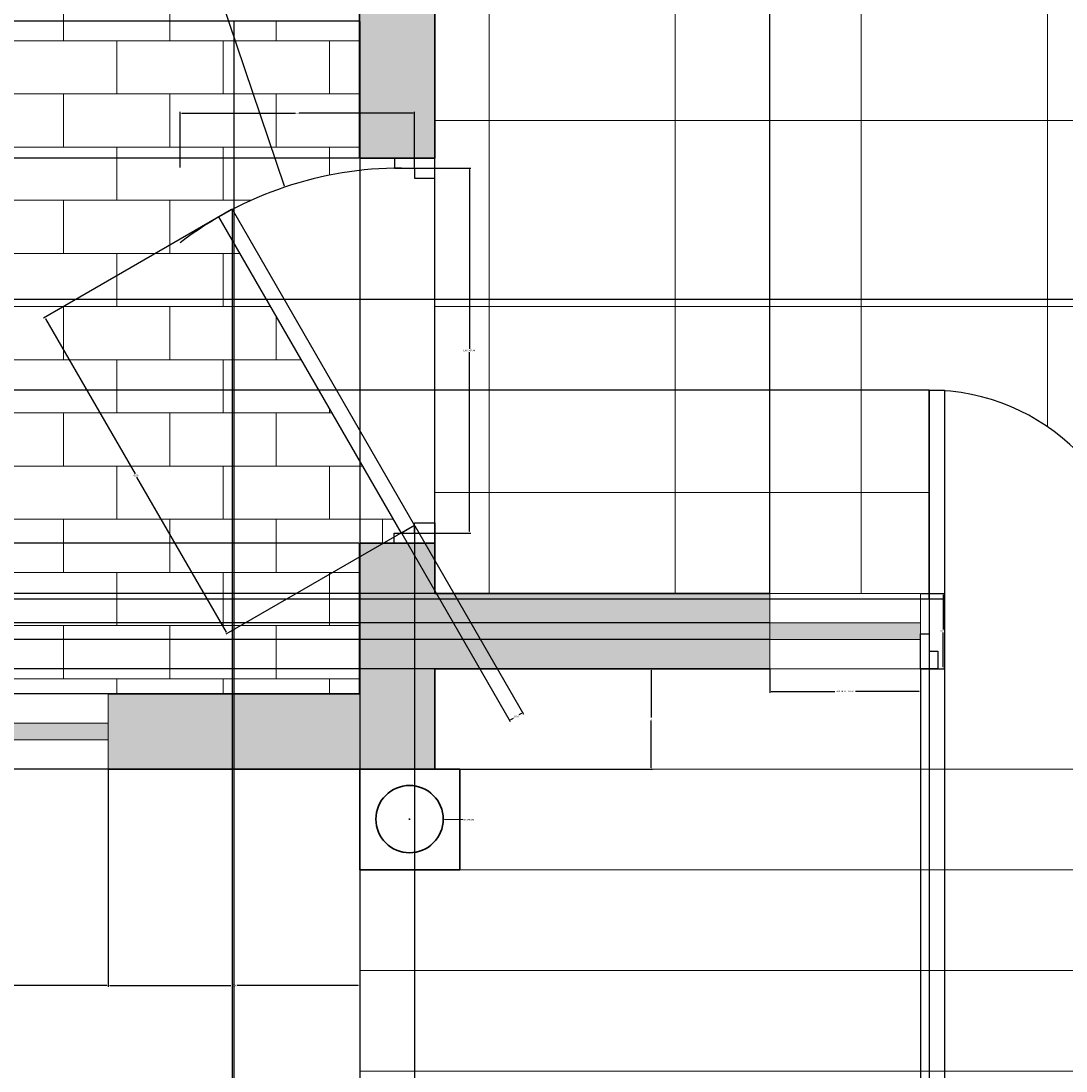
# Model space of a CAD drawing. Units: inches. Extents: x 6 to 575, y 34 to 566.
# Tile 4 of 21: x 157 to 282, y 168 to 293. Entities that reach past the tile are written whole.
import ezdxf

# ---------------------------------------------------------------- set-up
doc = ezdxf.new("R2010")
doc.units = ezdxf.units.IN
doc.linetypes.add('ACAD_ISO02W100', pattern=[15, 12, -3])
for name, color, linetype, lineweight in [('A-ANNO-DIMS', 2, 'Continuous', 18), ('A-COLS', 7, 'Continuous', 35), ('A-DOOR-THRS', 8, 'Continuous', 13), ('A-FLOR-PATT', 252, 'Continuous', 9), ('A-GLAZ-PATT', 4, 'Continuous', 9), ('A-ROOF-OVHD', 240, 'ACAD_ISO02W100', 13), ('A-WALL-PATT', 251, 'Continuous', 9), ('DOORS', 3, 'Continuous', 25), ('STAIRS', 1, 'Continuous', 20), ('WALLS', 7, 'Continuous', 35), ('WINDOWS', 4, 'Continuous', 20)]:
    doc.layers.add(name, color=color, linetype=linetype, lineweight=lineweight)
doc.styles.get("Standard").update_dxf_attribs({"font": 'arial.ttf'})
doc.dimstyles.get("Standard").update_dxf_attribs({"dimtxt": 0.18, "dimasz": 0.18, "dimexe": 0.18, "dimexo": 0.0625, "dimgap": 0.09, "dimtad": 0, "dimtih": 1, "dimtoh": 1, "dimdec": 4, "dimzin": 0, "dimdsep": 46, "dimtxsty": 'Standard', "dimcen": 0.09, "dimadec": 0, "dimazin": 0, "dimtfac": 1, "dimtdec": 4, "dimtofl": 0, "dimtmove": 0, "dimatfit": 3, "dimfxl": 1, "dimtolj": 1, "dimtzin": 0, "dimarcsym": 0})

# ---------------------------------------------------------------- blocks, each defined once
blk = doc.blocks.new('Door - Left Hung 36 in.')
blk.add_lwpolyline([(0.75, -1.3), (0, 0), (31.18, 18), (31.93, 16.7)], close=True)
blk.add_arc((0, 0), 36, 0, 37.3101)
blk = doc.blocks.new('*U4')
for p, q in [((0, 0), (0, -6)), ((24, 0), (24, -6))]:
    blk.add_line(p, q)
blk.add_lwpolyline([(0, 0), (0, 24), (1.75, 24), (1.75, 0)], close=True)
blk.add_arc((0, 0), 24, 0, 90)
blk = doc.blocks.new('WIN-SIDELIGHT-18IN')
for p, q in [((0, 9), (0, 0)), ((0, 0), (0, 9)), ((0, 9), (0, 0)), ((18, 9), (18, 0)), ((0, 5.5), (18, 5.5)), ((0, 3.5), (18, 3.5))]:
    blk.add_line(p, q)
blk.add_lwpolyline([(0, 9), (18, 9), (18, 0), (0, 0)], close=True)
blk = doc.blocks.new('COL-PORTICO-RECT-BASE')
blk.add_lwpolyline([(0, 12.01), (11.94, 12.01), (11.94, 0), (0, 0)], close=True)
blk.add_circle((5.95, 6.05), 4.02)
blk = doc.blocks.new('*D15')
at = {"layer": 'A-ANNO-DIMS', "color": 0, "lineweight": -2, "transparency": 16777216}
for p, q in [((204.3, 275.6), (210.96, 275.6)), ((210.78, 275.42), (210.78, 253.99)), ((210.78, 232.19), (210.78, 253.62)), ((204.3, 232.01), (210.96, 232.01))]:
    blk.add_line(p, q, dxfattribs=at)
at = {"layer": 'A-ANNO-DIMS', "color": 0, "transparency": 16777216}
for points in [[(210.75, 275.42), (210.81, 275.42), (210.78, 275.6)], [(210.75, 232.19), (210.81, 232.19), (210.78, 232.01)]]:
    blk.add_solid(points, dxfattribs=at)
at = {"layer": 'Defpoints', "color": 0, "transparency": 16777216}
for p in [(204.24, 275.6), (210.78, 275.6), (204.24, 232.01)]:
    blk.add_point(p, dxfattribs=at)
at = {"layer": 'A-ANNO-DIMS', "color": 0, "transparency": 16777216, "insert": (210.78, 253.81), "char_height": 0.18, "attachment_point": 5}
blk.add_mtext('\\A1;LH DOOR 44', dxfattribs=at)
blk = doc.blocks.new('*D16')
at = {"layer": 'A-ANNO-DIMS', "color": 0, "lineweight": -2, "transparency": 16777216}
for p, q in [((176.25, 275.66), (176.25, 282.32)), ((204.24, 275.66), (204.24, 282.32)), ((176.43, 282.14), (190.02, 282.14)), ((204.06, 282.14), (190.46, 282.14))]:
    blk.add_line(p, q, dxfattribs=at)
at = {"layer": 'A-ANNO-DIMS', "color": 0, "transparency": 16777216}
for points in [[(176.43, 282.17), (176.43, 282.11), (176.25, 282.14)], [(204.06, 282.17), (204.06, 282.11), (204.24, 282.14)]]:
    blk.add_solid(points, dxfattribs=at)
at = {"layer": 'Defpoints', "color": 0, "transparency": 16777216}
for p in [(176.25, 282.14), (176.25, 275.6), (204.24, 275.6)]:
    blk.add_point(p, dxfattribs=at)
at = {"layer": 'A-ANNO-DIMS', "color": 0, "transparency": 16777216, "insert": (190.24, 282.14), "char_height": 0.18, "attachment_point": 5}
blk.add_mtext('\\A1;28', dxfattribs=at)
blk = doc.blocks.new('*D19')
at = {"layer": 'A-ANNO-DIMS', "color": 0, "lineweight": -2, "transparency": 16777216}
for p, q in [((246.66, 215.74), (246.66, 212.92)), ((264.66, 215.74), (264.66, 212.92)), ((246.84, 213.1), (254.43, 213.1)), ((264.48, 213.1), (256.88, 213.1))]:
    blk.add_line(p, q, dxfattribs=at)
at = {"layer": 'A-ANNO-DIMS', "color": 0, "transparency": 16777216}
for points in [[(246.84, 213.13), (246.84, 213.07), (246.66, 213.1)], [(264.48, 213.13), (264.48, 213.07), (264.66, 213.1)]]:
    blk.add_solid(points, dxfattribs=at)
at = {"layer": 'Defpoints', "color": 0, "transparency": 16777216}
for p in [(246.66, 215.8), (264.66, 215.8), (264.66, 213.1)]:
    blk.add_point(p, dxfattribs=at)
at = {"layer": 'A-ANNO-DIMS', "color": 0, "transparency": 16777216, "insert": (255.66, 213.1), "char_height": 0.18, "attachment_point": 5}
blk.add_mtext('\\A1;SIDELIGHT 18 TYP.', dxfattribs=at)
blk = doc.blocks.new('*D20')
at = {"layer": 'A-ANNO-DIMS', "color": 0, "lineweight": -2, "transparency": 16777216}
for p, q in [((264.72, 224.8), (267.54, 224.8)), ((267.36, 224.62), (267.36, 220.48)), ((267.36, 215.98), (267.36, 220.12)), ((264.72, 215.8), (267.54, 215.8))]:
    blk.add_line(p, q, dxfattribs=at)
at = {"layer": 'A-ANNO-DIMS', "color": 0, "transparency": 16777216}
for points in [[(267.33, 224.62), (267.39, 224.62), (267.36, 224.8)], [(267.33, 215.98), (267.39, 215.98), (267.36, 215.8)]]:
    blk.add_solid(points, dxfattribs=at)
at = {"layer": 'Defpoints', "color": 0, "transparency": 16777216}
for p in [(264.66, 224.8), (267.36, 224.8), (264.66, 215.8)]:
    blk.add_point(p, dxfattribs=at)
at = {"layer": 'A-ANNO-DIMS', "color": 0, "transparency": 16777216, "insert": (267.36, 220.3), "char_height": 0.18, "attachment_point": 5}
blk.add_mtext('\\A1;9 TYP.', dxfattribs=at)
blk = doc.blocks.new('*D29')
at = {"layer": 'A-ANNO-DIMS', "color": 0, "lineweight": -2, "transparency": 16777216}
for p, q in [((32.66, 203.74), (32.66, 33.76)), ((548.66, 203.74), (548.66, 33.76)), ((32.84, 33.94), (290.37, 33.94)), ((548.48, 33.94), (290.95, 33.94))]:
    blk.add_line(p, q, dxfattribs=at)
at = {"layer": 'A-ANNO-DIMS', "color": 0, "transparency": 16777216}
for points in [[(32.84, 33.97), (32.84, 33.91), (32.66, 33.94)], [(548.48, 33.97), (548.48, 33.91), (548.66, 33.94)]]:
    blk.add_solid(points, dxfattribs=at)
at = {"layer": 'Defpoints', "color": 0, "transparency": 16777216}
for p in [(32.66, 203.8), (548.66, 203.8), (548.66, 33.94)]:
    blk.add_point(p, dxfattribs=at)
at = {"layer": 'A-ANNO-DIMS', "color": 0, "transparency": 16777216, "insert": (290.66, 33.94), "char_height": 0.18, "attachment_point": 5}
blk.add_mtext('\\A1;516', dxfattribs=at)
blk = doc.blocks.new('*D30')
at = {"layer": 'A-ANNO-DIMS', "color": 0, "lineweight": -2, "transparency": 16777216}
for p, q in [((32.6, 539.8), (6.65, 539.8)), ((6.83, 539.62), (6.83, 299.97)), ((6.83, 59.95), (6.83, 299.61)), ((197.62, 59.77), (6.65, 59.77))]:
    blk.add_line(p, q, dxfattribs=at)
at = {"layer": 'A-ANNO-DIMS', "color": 0, "transparency": 16777216}
for points in [[(6.8, 539.62), (6.86, 539.62), (6.83, 539.8)], [(6.8, 59.95), (6.86, 59.95), (6.83, 59.77)]]:
    blk.add_solid(points, dxfattribs=at)
at = {"layer": 'Defpoints', "color": 0, "transparency": 16777216}
for p in [(32.66, 539.8), (6.83, 59.77), (197.69, 59.77)]:
    blk.add_point(p, dxfattribs=at)
at = {"layer": 'A-ANNO-DIMS', "color": 0, "transparency": 16777216, "insert": (6.83, 299.79), "char_height": 0.18, "attachment_point": 5}
blk.add_mtext('\\A1;480', dxfattribs=at)
blk = doc.blocks.new('*D37')
at = {"layer": 'A-ANNO-DIMS', "color": 0, "lineweight": -2, "transparency": 16777216}
for p, q in [((71.66, 203.74), (71.66, 177.79)), ((167.66, 203.74), (167.66, 177.79)), ((71.84, 177.97), (119.44, 177.97)), ((167.48, 177.97), (119.88, 177.97))]:
    blk.add_line(p, q, dxfattribs=at)
at = {"layer": 'A-ANNO-DIMS', "color": 0, "transparency": 16777216}
for points in [[(71.84, 178), (71.84, 177.94), (71.66, 177.97)], [(167.48, 178), (167.48, 177.94), (167.66, 177.97)]]:
    blk.add_solid(points, dxfattribs=at)
at = {"layer": 'Defpoints', "color": 0, "transparency": 16777216}
for p in [(71.66, 203.8), (167.66, 203.8), (71.66, 177.97)]:
    blk.add_point(p, dxfattribs=at)
at = {"layer": 'A-ANNO-DIMS', "color": 0, "transparency": 16777216, "insert": (119.66, 177.97), "char_height": 0.18, "attachment_point": 5}
blk.add_mtext('\\A1;96', dxfattribs=at)
blk = doc.blocks.new('*D39')
at = {"layer": 'A-ANNO-DIMS', "color": 0, "lineweight": -2, "transparency": 16777216}
for p, q in [((167.66, 203.74), (167.66, 177.79)), ((197.69, 203.74), (197.69, 177.79)), ((167.84, 177.97), (182.28, 177.97)), ((197.51, 177.97), (183.07, 177.97))]:
    blk.add_line(p, q, dxfattribs=at)
at = {"layer": 'A-ANNO-DIMS', "color": 0, "transparency": 16777216}
for points in [[(167.84, 178), (167.84, 177.94), (167.66, 177.97)], [(197.51, 178), (197.51, 177.94), (197.69, 177.97)]]:
    blk.add_solid(points, dxfattribs=at)
at = {"layer": 'Defpoints', "color": 0, "transparency": 16777216}
for p in [(167.66, 203.8), (197.69, 203.8), (167.66, 177.97)]:
    blk.add_point(p, dxfattribs=at)
at = {"layer": 'A-ANNO-DIMS', "color": 0, "transparency": 16777216, "insert": (182.67, 177.97), "char_height": 0.18, "attachment_point": 5}
blk.add_mtext('\\A1;30.03', dxfattribs=at)
blk = doc.blocks.new('*D48')
at = {"layer": 'A-ANNO-DIMS', "color": 0, "lineweight": -2, "transparency": 16777216}
for p, q in [((264.66, 215.74), (264.66, 33.76)), ((316.66, 215.74), (316.66, 33.76)), ((264.84, 33.94), (290.44, 33.94)), ((316.48, 33.94), (290.88, 33.94))]:
    blk.add_line(p, q, dxfattribs=at)
at = {"layer": 'A-ANNO-DIMS', "color": 0, "transparency": 16777216}
for points in [[(264.84, 33.97), (264.84, 33.91), (264.66, 33.94)], [(316.48, 33.97), (316.48, 33.91), (316.66, 33.94)]]:
    blk.add_solid(points, dxfattribs=at)
at = {"layer": 'Defpoints', "color": 0, "transparency": 16777216}
for p in [(264.66, 215.8), (316.66, 215.8), (316.66, 33.94)]:
    blk.add_point(p, dxfattribs=at)
at = {"layer": 'A-ANNO-DIMS', "color": 0, "transparency": 16777216, "insert": (290.66, 33.94), "char_height": 0.18, "attachment_point": 5}
blk.add_mtext('\\A1;52', dxfattribs=at)
blk = doc.blocks.new('*D54')
at = {"layer": 'A-ANNO-DIMS', "color": 0, "lineweight": -2, "transparency": 16777216}
for p, q in [((444.96, 337.94), (6.65, 337.94)), ((6.83, 337.76), (6.83, 299.11)), ((6.83, 260.1), (6.83, 298.75)), ((444.96, 259.92), (6.65, 259.92))]:
    blk.add_line(p, q, dxfattribs=at)
at = {"layer": 'A-ANNO-DIMS', "color": 0, "transparency": 16777216}
for points in [[(6.8, 337.76), (6.86, 337.76), (6.83, 337.94)], [(6.8, 260.1), (6.86, 260.1), (6.83, 259.92)]]:
    blk.add_solid(points, dxfattribs=at)
at = {"layer": 'Defpoints', "color": 0, "transparency": 16777216}
for p in [(6.83, 337.94), (445.02, 337.94), (445.02, 259.92)]:
    blk.add_point(p, dxfattribs=at)
at = {"layer": 'A-ANNO-DIMS', "color": 0, "transparency": 16777216, "insert": (6.83, 298.93), "char_height": 0.18, "attachment_point": 5}
blk.add_mtext('\\A1;78.02', dxfattribs=at)
blk = doc.blocks.new('*D59')
at = {"layer": 'A-ANNO-DIMS', "color": 0, "lineweight": -2, "transparency": 16777216}
for p, q in [((206.66, 224.86), (206.66, 565.81)), ((206.84, 565.63), (226.44, 565.63)), ((246.48, 565.63), (226.88, 565.63)), ((246.66, 224.86), (246.66, 565.81))]:
    blk.add_line(p, q, dxfattribs=at)
at = {"layer": 'A-ANNO-DIMS', "color": 0, "transparency": 16777216}
for points in [[(206.84, 565.66), (206.84, 565.6), (206.66, 565.63)], [(246.48, 565.66), (246.48, 565.6), (246.66, 565.63)]]:
    blk.add_solid(points, dxfattribs=at)
at = {"layer": 'Defpoints', "color": 0, "transparency": 16777216}
for p in [(246.66, 565.63), (206.66, 224.8), (246.66, 224.8)]:
    blk.add_point(p, dxfattribs=at)
at = {"layer": 'A-ANNO-DIMS', "color": 0, "transparency": 16777216, "insert": (226.66, 565.63), "char_height": 0.18, "attachment_point": 5}
blk.add_mtext('\\A1;40', dxfattribs=at)
blk = doc.blocks.new('*D60')
at = {"layer": 'A-ANNO-DIMS', "color": 0, "lineweight": -2, "transparency": 16777216}
for p, q in [((206.72, 215.8), (232.67, 215.8)), ((232.49, 215.62), (232.49, 209.98)), ((232.49, 203.98), (232.49, 209.62)), ((206.72, 203.8), (232.67, 203.8))]:
    blk.add_line(p, q, dxfattribs=at)
at = {"layer": 'A-ANNO-DIMS', "color": 0, "transparency": 16777216}
for points in [[(232.46, 215.62), (232.52, 215.62), (232.49, 215.8)], [(232.46, 203.98), (232.52, 203.98), (232.49, 203.8)]]:
    blk.add_solid(points, dxfattribs=at)
at = {"layer": 'Defpoints', "color": 0, "transparency": 16777216}
for p in [(206.66, 215.8), (206.66, 203.8), (232.49, 203.8)]:
    blk.add_point(p, dxfattribs=at)
at = {"layer": 'A-ANNO-DIMS', "color": 0, "transparency": 16777216, "insert": (232.49, 209.8), "char_height": 0.18, "attachment_point": 5}
blk.add_mtext('\\A1;12', dxfattribs=at)
blk = doc.blocks.new('*D77')
at = {"layer": 'A-ANNO-DIMS', "color": 0, "lineweight": -2, "transparency": 16777216}
for p, q in [((197.62, 203.8), (6.65, 203.8)), ((6.83, 203.62), (6.83, 131.97)), ((6.83, 59.95), (6.83, 131.61)), ((197.62, 59.77), (6.65, 59.77))]:
    blk.add_line(p, q, dxfattribs=at)
at = {"layer": 'A-ANNO-DIMS', "color": 0, "transparency": 16777216}
for points in [[(6.8, 203.62), (6.86, 203.62), (6.83, 203.8)], [(6.8, 59.95), (6.86, 59.95), (6.83, 59.77)]]:
    blk.add_solid(points, dxfattribs=at)
at = {"layer": 'Defpoints', "color": 0, "transparency": 16777216}
for p in [(6.83, 203.8), (197.69, 203.8), (197.69, 59.77)]:
    blk.add_point(p, dxfattribs=at)
at = {"layer": 'A-ANNO-DIMS', "color": 0, "transparency": 16777216, "insert": (6.83, 131.79), "char_height": 0.18, "attachment_point": 5}
blk.add_mtext('\\A1;144.03', dxfattribs=at)
blk = doc.blocks.new('*D104')
at = {"layer": 'A-ANNO-DIMS', "color": 0, "lineweight": -2, "transparency": 16777216}
for p, q in [((197.64, 348.32), (6.65, 348.32)), ((6.83, 348.14), (6.83, 320.93)), ((6.83, 293.34), (6.83, 320.56)), ((182.58, 293.16), (6.65, 293.16))]:
    blk.add_line(p, q, dxfattribs=at)
at = {"layer": 'A-ANNO-DIMS', "color": 0, "transparency": 16777216}
for points in [[(6.8, 348.14), (6.86, 348.14), (6.83, 348.32)], [(6.8, 293.34), (6.86, 293.34), (6.83, 293.16)]]:
    blk.add_solid(points, dxfattribs=at)
at = {"layer": 'Defpoints', "color": 0, "transparency": 16777216}
for p in [(6.83, 348.32), (197.7, 348.32), (182.64, 293.16)]:
    blk.add_point(p, dxfattribs=at)
at = {"layer": 'A-ANNO-DIMS', "color": 0, "transparency": 16777216, "insert": (6.83, 320.74), "char_height": 0.18, "attachment_point": 5}
blk.add_mtext('\\A1;55.16', dxfattribs=at)
blk = doc.blocks.new('*D105')
at = {"layer": 'A-ANNO-DIMS', "color": 0, "lineweight": -2, "transparency": 16777216}
for p, q in [((182.64, 293.1), (182.64, 33.76)), ((197.7, 293.1), (197.7, 33.76)), ((182.82, 33.94), (189.71, 33.94)), ((197.52, 33.94), (190.62, 33.94))]:
    blk.add_line(p, q, dxfattribs=at)
at = {"layer": 'A-ANNO-DIMS', "color": 0, "transparency": 16777216}
for points in [[(182.82, 33.97), (182.82, 33.91), (182.64, 33.94)], [(197.52, 33.97), (197.52, 33.91), (197.7, 33.94)]]:
    blk.add_solid(points, dxfattribs=at)
at = {"layer": 'Defpoints', "color": 0, "transparency": 16777216}
for p in [(182.64, 293.16), (197.7, 293.16), (197.7, 33.94)]:
    blk.add_point(p, dxfattribs=at)
at = {"layer": 'A-ANNO-DIMS', "color": 0, "transparency": 16777216, "insert": (190.17, 33.94), "char_height": 0.18, "attachment_point": 5}
blk.add_mtext('\\A1;15.058', dxfattribs=at)
blk = doc.blocks.new('*D106')
at = {"layer": 'A-ANNO-DIMS', "color": 0, "lineweight": -2, "transparency": 16777216}
for p, q in [((197.64, 293.16), (6.65, 293.16)), ((6.83, 292.98), (6.83, 285.16)), ((6.83, 276.98), (6.83, 284.8)), ((197.6, 276.8), (6.65, 276.8))]:
    blk.add_line(p, q, dxfattribs=at)
at = {"layer": 'A-ANNO-DIMS', "color": 0, "transparency": 16777216}
for points in [[(6.8, 292.98), (6.86, 292.98), (6.83, 293.16)], [(6.8, 276.98), (6.86, 276.98), (6.83, 276.8)]]:
    blk.add_solid(points, dxfattribs=at)
at = {"layer": 'Defpoints', "color": 0, "transparency": 16777216}
for p in [(6.83, 293.16), (197.7, 293.16), (197.66, 276.8)]:
    blk.add_point(p, dxfattribs=at)
at = {"layer": 'A-ANNO-DIMS', "color": 0, "transparency": 16777216, "insert": (6.83, 284.98), "char_height": 0.18, "attachment_point": 5}
blk.add_mtext('\\A1;16.363', dxfattribs=at)
blk = doc.blocks.new('*D107')
at = {"layer": 'A-ANNO-DIMS', "color": 0, "lineweight": -2, "transparency": 16777216}
for p, q in [((197.6, 230.8), (6.65, 230.8)), ((6.83, 230.62), (6.83, 221.98)), ((6.83, 212.98), (6.83, 221.62)), ((197.6, 212.8), (6.65, 212.8))]:
    blk.add_line(p, q, dxfattribs=at)
at = {"layer": 'A-ANNO-DIMS', "color": 0, "transparency": 16777216}
for points in [[(6.8, 230.62), (6.86, 230.62), (6.83, 230.8)], [(6.8, 212.98), (6.86, 212.98), (6.83, 212.8)]]:
    blk.add_solid(points, dxfattribs=at)
at = {"layer": 'Defpoints', "color": 0, "transparency": 16777216}
for p in [(6.83, 230.8), (197.66, 230.8), (197.66, 212.8)]:
    blk.add_point(p, dxfattribs=at)
at = {"layer": 'A-ANNO-DIMS', "color": 0, "transparency": 16777216, "insert": (6.83, 221.8), "char_height": 0.18, "attachment_point": 5}
blk.add_mtext('\\A1;18', dxfattribs=at)
blk = doc.blocks.new('*D108')
at = {"layer": 'A-ANNO-DIMS', "color": 0, "lineweight": -2, "transparency": 16777216}
for p, q in [((197.6, 276.8), (6.65, 276.8)), ((6.83, 276.62), (6.83, 253.98)), ((6.83, 230.98), (6.83, 253.62)), ((197.6, 230.8), (6.65, 230.8))]:
    blk.add_line(p, q, dxfattribs=at)
at = {"layer": 'A-ANNO-DIMS', "color": 0, "transparency": 16777216}
for points in [[(6.8, 276.62), (6.86, 276.62), (6.83, 276.8)], [(6.8, 230.98), (6.86, 230.98), (6.83, 230.8)]]:
    blk.add_solid(points, dxfattribs=at)
at = {"layer": 'Defpoints', "color": 0, "transparency": 16777216}
for p in [(6.83, 276.8), (197.66, 276.8), (197.66, 230.8)]:
    blk.add_point(p, dxfattribs=at)
at = {"layer": 'A-ANNO-DIMS', "color": 0, "transparency": 16777216, "insert": (6.83, 253.8), "char_height": 0.18, "attachment_point": 5}
blk.add_mtext('\\A1;46', dxfattribs=at)
blk = doc.blocks.new('*D137')
at = {"layer": 'A-ANNO-DIMS', "color": 0, "lineweight": -2, "transparency": 16777216}
for p, q in [((206.62, 310.57), (6.65, 310.57)), ((6.83, 310.39), (6.83, 267.87)), ((6.83, 224.98), (6.83, 267.5)), ((206.6, 224.8), (6.65, 224.8))]:
    blk.add_line(p, q, dxfattribs=at)
at = {"layer": 'A-ANNO-DIMS', "color": 0, "transparency": 16777216}
for points in [[(6.8, 310.39), (6.86, 310.39), (6.83, 310.57)], [(6.8, 224.98), (6.86, 224.98), (6.83, 224.8)]]:
    blk.add_solid(points, dxfattribs=at)
at = {"layer": 'Defpoints', "color": 0, "transparency": 16777216}
for p in [(6.83, 310.57), (206.68, 310.57), (206.66, 224.8)]:
    blk.add_point(p, dxfattribs=at)
at = {"layer": 'A-ANNO-DIMS', "color": 0, "transparency": 16777216, "insert": (6.83, 267.69), "char_height": 0.18, "attachment_point": 5}
blk.add_mtext('\\A1;85.77', dxfattribs=at)
blk = doc.blocks.new('*D206')
at = {"layer": 'A-ANNO-DIMS', "color": 0, "lineweight": -2, "transparency": 16777216}
for p, q in [((182.39, 270.64), (159.92, 257.66)), ((160.16, 257.6), (170.87, 239.06)), ((181.78, 220.16), (171.08, 238.7)), ((204.18, 232.89), (181.71, 219.91))]:
    blk.add_line(p, q, dxfattribs=at)
at = {"layer": 'A-ANNO-DIMS', "color": 0, "transparency": 16777216}
for points in [[(160.19, 257.61), (160.14, 257.58), (160.07, 257.75)], [(181.8, 220.18), (181.75, 220.15), (181.87, 220)]]:
    blk.add_solid(points, dxfattribs=at)
at = {"layer": 'Defpoints', "color": 0, "transparency": 16777216}
for p in [(182.44, 270.67), (160.07, 257.75), (204.24, 232.92)]:
    blk.add_point(p, dxfattribs=at)
at = {"layer": 'A-ANNO-DIMS', "color": 0, "transparency": 16777216, "insert": (170.97, 238.88), "char_height": 0.18, "attachment_point": 5}
blk.add_mtext('\\A1;43.59', dxfattribs=at)
blk = doc.blocks.new('*D207')
at = {"layer": 'A-ANNO-DIMS', "color": 0, "lineweight": -2, "transparency": 16777216}
for p, q in [((204.27, 232.87), (217.24, 210.39)), ((202.7, 231.96), (215.67, 209.49)), ((215.74, 209.73), (216.05, 209.91)), ((217, 210.46), (216.68, 210.28))]:
    blk.add_line(p, q, dxfattribs=at)
at = {"layer": 'A-ANNO-DIMS', "color": 0, "transparency": 16777216}
for points in [[(215.72, 209.76), (215.75, 209.71), (215.58, 209.64)], [(216.98, 210.49), (217.01, 210.43), (217.15, 210.55)]]:
    blk.add_solid(points, dxfattribs=at)
at = {"layer": 'Defpoints', "color": 0, "transparency": 16777216}
for p in [(202.66, 232.01), (204.24, 232.92), (215.58, 209.64)]:
    blk.add_point(p, dxfattribs=at)
at = {"layer": 'A-ANNO-DIMS', "color": 0, "transparency": 16777216, "insert": (216.37, 210.1), "char_height": 0.18, "attachment_point": 5}
blk.add_mtext('\\A1;1.816', dxfattribs=at)
blk = doc.blocks.new('*D208')
at = {"layer": 'A-ANNO-DIMS', "color": 0, "lineweight": -2, "transparency": 16777216}
for p, q in [((182.44, 270.6), (182.44, 33.76)), ((204.24, 232.86), (204.24, 33.76)), ((182.62, 33.94), (192.88, 33.94)), ((204.06, 33.94), (193.81, 33.94))]:
    blk.add_line(p, q, dxfattribs=at)
at = {"layer": 'A-ANNO-DIMS', "color": 0, "transparency": 16777216}
for points in [[(182.62, 33.97), (182.62, 33.91), (182.44, 33.94)], [(204.06, 33.97), (204.06, 33.91), (204.24, 33.94)]]:
    blk.add_solid(points, dxfattribs=at)
at = {"layer": 'Defpoints', "color": 0, "transparency": 16777216}
for p in [(182.44, 270.67), (204.24, 232.92), (182.44, 33.94)]:
    blk.add_point(p, dxfattribs=at)
at = {"layer": 'A-ANNO-DIMS', "color": 0, "transparency": 16777216, "insert": (193.34, 33.94), "char_height": 0.18, "attachment_point": 5}
blk.add_mtext('\\A1;21.793', dxfattribs=at)
blk = doc.blocks.new('*D209')
at = {"layer": 'A-ANNO-DIMS', "color": 0, "lineweight": -2, "transparency": 16777216}
for p, q in [((265.64, 249.08), (6.65, 249.08)), ((6.83, 248.9), (6.83, 236.78)), ((6.83, 224.3), (6.83, 236.42)), ((265.64, 224.12), (6.65, 224.12))]:
    blk.add_line(p, q, dxfattribs=at)
at = {"layer": 'A-ANNO-DIMS', "color": 0, "transparency": 16777216}
for points in [[(6.8, 248.9), (6.86, 248.9), (6.83, 249.08)], [(6.8, 224.3), (6.86, 224.3), (6.83, 224.12)]]:
    blk.add_solid(points, dxfattribs=at)
at = {"layer": 'Defpoints', "color": 0, "transparency": 16777216}
for p in [(6.83, 249.08), (265.7, 249.08), (265.7, 224.12)]:
    blk.add_point(p, dxfattribs=at)
at = {"layer": 'A-ANNO-DIMS', "color": 0, "transparency": 16777216, "insert": (6.83, 236.6), "char_height": 0.18, "attachment_point": 5}
blk.add_mtext('\\A1;24.96', dxfattribs=at)
blk = doc.blocks.new('*D210')
at = {"layer": 'A-ANNO-DIMS', "color": 0, "lineweight": -2, "transparency": 16777216}
for p, q in [((265.7, 249.02), (265.7, 33.76)), ((267.52, 249.02), (267.52, 33.76)), ((265.88, 33.94), (266.29, 33.94)), ((267.34, 33.94), (266.92, 33.94))]:
    blk.add_line(p, q, dxfattribs=at)
at = {"layer": 'A-ANNO-DIMS', "color": 0, "transparency": 16777216}
for points in [[(265.88, 33.97), (265.88, 33.91), (265.7, 33.94)], [(267.34, 33.97), (267.34, 33.91), (267.52, 33.94)]]:
    blk.add_solid(points, dxfattribs=at)
at = {"layer": 'Defpoints', "color": 0, "transparency": 16777216}
for p in [(265.7, 249.08), (267.52, 249.08), (267.52, 33.94)]:
    blk.add_point(p, dxfattribs=at)
at = {"layer": 'A-ANNO-DIMS', "color": 0, "transparency": 16777216, "insert": (266.61, 33.94), "char_height": 0.18, "attachment_point": 5}
blk.add_mtext('\\A1;1.82', dxfattribs=at)
blk = doc.blocks.new('*D214')
at = {"layer": 'A-ANNO-DIMS', "color": 0, "lineweight": -2, "transparency": 16777216}
for p, q in [((246.6, 219.3), (6.65, 219.3)), ((6.83, 219.12), (6.83, 217.73)), ((6.83, 215.98), (6.83, 217.37)), ((246.6, 215.8), (6.65, 215.8))]:
    blk.add_line(p, q, dxfattribs=at)
at = {"layer": 'A-ANNO-DIMS', "color": 0, "transparency": 16777216}
for points in [[(6.8, 219.12), (6.86, 219.12), (6.83, 219.3)], [(6.8, 215.98), (6.86, 215.98), (6.83, 215.8)]]:
    blk.add_solid(points, dxfattribs=at)
at = {"layer": 'Defpoints', "color": 0, "transparency": 16777216}
for p in [(6.83, 219.3), (246.66, 219.3), (246.66, 215.8)]:
    blk.add_point(p, dxfattribs=at)
at = {"layer": 'A-ANNO-DIMS', "color": 0, "transparency": 16777216, "insert": (6.83, 217.55), "char_height": 0.18, "attachment_point": 5}
blk.add_mtext('\\A1;3.5', dxfattribs=at)
blk = doc.blocks.new('*D215')
at = {"layer": 'A-ANNO-DIMS', "color": 0, "lineweight": -2, "transparency": 16777216}
for p, q in [((246.6, 221.3), (6.65, 221.3)), ((6.83, 221.12), (6.83, 220.48)), ((6.83, 219.48), (6.83, 220.12)), ((246.6, 219.3), (6.65, 219.3))]:
    blk.add_line(p, q, dxfattribs=at)
at = {"layer": 'A-ANNO-DIMS', "color": 0, "transparency": 16777216}
for points in [[(6.8, 221.12), (6.86, 221.12), (6.83, 221.3)], [(6.8, 219.48), (6.86, 219.48), (6.83, 219.3)]]:
    blk.add_solid(points, dxfattribs=at)
at = {"layer": 'Defpoints', "color": 0, "transparency": 16777216}
for p in [(6.83, 221.3), (246.66, 221.3), (246.66, 219.3)]:
    blk.add_point(p, dxfattribs=at)
at = {"layer": 'A-ANNO-DIMS', "color": 0, "transparency": 16777216, "insert": (6.83, 220.3), "char_height": 0.18, "attachment_point": 5}
blk.add_mtext('\\A1;2', dxfattribs=at)
blk = doc.blocks.new('*D219')
at = {"layer": 'A-ANNO-DIMS', "color": 0, "lineweight": -2, "transparency": 16777216}
for p, q in [((203.54, 197.84), (203.72, 197.84)), ((203.63, 197.75), (203.63, 197.93)), ((210.06, 197.76), (207.83, 197.79))]:
    blk.add_line(p, q, dxfattribs=at)
at = {"layer": 'A-ANNO-DIMS', "color": 0, "transparency": 16777216}
blk.add_solid([(207.83, 197.82), (207.83, 197.76), (207.65, 197.79)], dxfattribs=at)
at = {"layer": 'Defpoints', "color": 0, "transparency": 16777216}
for p in [(199.62, 197.89), (207.65, 197.79)]:
    blk.add_point(p, dxfattribs=at)
at = {"layer": 'A-ANNO-DIMS', "color": 0, "transparency": 16777216, "insert": (210.74, 197.76), "char_height": 0.18, "attachment_point": 5}
blk.add_mtext('\\A1;4X ∅8.036', dxfattribs=at)
blk = doc.blocks.new('*D228')
at = {"layer": 'A-ANNO-DIMS', "color": 0, "lineweight": -2, "transparency": 16777216}
for p, q in [((180.18, 298.09), (180.36, 298.09)), ((180.36, 298.09), (188.66, 273.48)), ((202.57, 232.01), (202.75, 232.01)), ((202.66, 231.92), (202.66, 232.1))]:
    blk.add_line(p, q, dxfattribs=at)
at = {"layer": 'A-ANNO-DIMS', "color": 0, "transparency": 16777216}
blk.add_solid([(188.69, 273.49), (188.64, 273.47), (188.72, 273.31)], dxfattribs=at)
at = {"layer": 'Defpoints', "color": 0, "transparency": 16777216}
for p in [(188.72, 273.31), (202.66, 232.01)]:
    blk.add_point(p, dxfattribs=at)
at = {"layer": 'A-ANNO-DIMS', "color": 0, "transparency": 16777216, "insert": (179.7, 298.09), "char_height": 0.18, "attachment_point": 5}
blk.add_mtext('\\A1;R43.59', dxfattribs=at)

msp = doc.modelspace()

# ---------------------------------------------------------------- hatches: boundary and pattern name
at = {"layer": 'A-FLOR-PATT'}
h = msp.add_hatch(dxfattribs=at)
h.set_pattern_fill('BRICK', color=256)
h.set_pattern_definition([(0, (-98.035, 170.1465), (0, 6.35), []), (90, (-98.035, 170.147), (-12.7, 8e-16), [6.35, -6.35]), (90, (-91.685, 170.147), (-12.7, 8e-16), [-6.35, 6.35])])
h.paths.add_polyline_path([(180.8711, 269.7588), (182.4439, 270.6668), (182.4628, 270.6341, -0.11619827), (201.8275, 275.5902), (201.8275, 276.801), (197.6586, 276.801), (197.6586, 293.1641), (182.6401, 293.1641), (182.6401, 348.324), (197.6586, 348.324), (197.6586, 407.7709), (112.8513, 407.7709), (112.8513, 431.801), (111.6586, 431.801), (111.6586, 440.801), (117.6586, 440.801), (117.6586, 446.801), (117.6586, 448.2751), (117.6586, 473.3269), (117.6586, 474.801), (117.6586, 515.5941), (100.2533, 515.5941, -1), (83.0548, 515.5941), (65.6494, 515.5941), (65.6494, 440.801), (82.8918, 440.801), (82.8918, 431.801), (82.8918, 407.7709), (41.6586, 407.7709), (41.6586, 379.0637), (62.6459, 379.0637), (62.6459, 358.0764), (122.565, 358.0764), (122.565, 286.0643), (62.6459, 286.0643), (62.6459, 265.077), (41.6586, 265.077), (41.6586, 224.801), (41.6586, 212.801), (71.6586, 212.801), (167.6586, 212.801), (197.6586, 212.801), (197.6586, 230.801), (201.8157, 230.801), (201.8157, 233.4817)])
h.paths.add_polyline_path([(133.3414, 245.1275), (133.3317, 245.1352), (133.3317, 245.104)], flags=16)
h.paths.add_polyline_path([(133.3317, 222.1662), (85.3496, 222.1662), (85.3496, 243.7443, -0.50090726), (87.1831, 246.1963), (107.4292, 246.1963), (111.2522, 246.1963), (131.4202, 246.1963, -0.41421356), (133.3317, 244.2848)], flags=16)
h.paths.add_polyline_path([(72.7105, 244.4018), (72.7105, 220.3718), (48.6804, 220.3718), (48.6804, 244.4018)], flags=16)
h.paths.add_polyline_path([(71.7466, 237.8955, -1), (59.8096, 237.8955, -1)], flags=0)
h = msp.add_hatch(dxfattribs=at)
h.set_pattern_fill('NET', color=256, scale=7)
h.set_pattern_definition([(0, (-98.035, 170.147), (0, 22.225), []), (90, (-98.035, 170.147), (-22.225, 1e-15), [])])
h.paths.add_polyline_path([(368.183, 395.6385, -0.88370529), (374.2533, 394.8861), (374.6586, 448.801), (354.6586, 448.801), (354.6586, 448.7938), (353.1847, 448.7938), (326.6586, 448.801), (322.6586, 448.801), (248.6332, 448.8024), (206.6586, 448.8024), (206.6586, 389.449), (221.6622, 389.449), (221.6622, 310.5712), (206.6586, 310.5712), (206.6586, 276.801), (206.6704, 276.801), (206.6704, 274.3795), (206.6586, 224.801), (246.6586, 224.801), (264.6586, 224.801), (265.6986, 224.801), (265.6986, 249.081), (267.5186, 249.081), (267.5186, 249.0145, -0.38515288), (290.6494, 224.801), (290.6679, 224.801, -0.38515288), (313.7986, 249.0145), (313.7986, 249.081), (315.6186, 249.081), (315.6186, 224.801), (316.6586, 224.801), (334.6586, 224.801), (374.6586, 224.801), (374.6586, 278.801), (374.1753, 318.8919, -0.45530286), (370.7577, 315.9168), (370.6643, 313.8205, -0.41421356), (368.7528, 311.909), (368.8072, 311.8975), (368.7528, 311.909, 0.41421356), (370.6643, 313.8205), (370.7632, 315.9161, -0.34634601), (368.183, 318.5897)])
h.paths.add_polyline_path([(288.603, 342.0131), (288.603, 389.9952), (318.6406, 389.9952), (318.6406, 342.0131)], flags=16)
h.paths.add_polyline_path([(289.6173, 343.0274), (289.6173, 389.059), (317.6263, 389.059), (317.6263, 343.0274)], flags=0)
h.paths.add_polyline_path([(295.4867, 311.7535, 0.06538163), (295.1241, 312.0945), (295.0006, 312.1316)], flags=16)
h.paths.add_polyline_path([(328.4931, 284.9911, 0.41421356), (330.4045, 286.9026), (330.4215, 286.8532), (330.4045, 286.9026, -0.41421356), (328.4931, 284.9911), (328.549, 284.9808)], flags=16)
h.paths.add_polyline_path([(344.7771, 305.2659), (368.8072, 305.2659), (368.8072, 281.2358), (344.7771, 281.2358)], flags=16)
h.paths.add_polyline_path([(368.183, 288.1406, -1), (356.246, 288.1406, -1)], flags=0)
h.paths.add_polyline_path([(347.9759, 404.6629), (347.9759, 428.6929), (372.006, 428.6929), (372.006, 404.6629)], flags=16)
h.paths.add_polyline_path([(359.4448, 421.7882, -1), (371.3818, 421.7882, -1)], flags=0)
at = {"layer": 'A-GLAZ-PATT'}
h = msp.add_hatch(color=256, dxfattribs=at)
h.dxf.hatch_style = 1
h.paths.add_polyline_path([(36.1586, 224.801), (38.1586, 224.801), (38.1586, 272.801), (36.1586, 272.801)])
h.paths.add_polyline_path([(167.6586, 207.301), (167.6586, 209.301), (71.6586, 209.301), (71.6586, 207.301)])
h.paths.add_polyline_path([(264.6586, 219.301), (264.6586, 221.301), (246.6586, 221.301), (246.6586, 219.301)])
h.paths.add_polyline_path([(316.6586, 221.301), (316.6586, 219.301), (334.6586, 219.301), (334.6586, 221.301)])
h.paths.add_polyline_path([(515.6586, 207.301), (515.6586, 209.301), (407.6586, 209.301), (407.6586, 207.301)])
h.paths.add_polyline_path([(543.1586, 270.801), (545.1586, 270.801), (545.1586, 366.801), (543.1586, 366.801)])
h.paths.add_polyline_path([(407.9436, 536.301), (407.9436, 534.301), (455.9436, 534.301), (455.9436, 536.301)])
h.paths.add_polyline_path([(272.6586, 536.301), (272.6586, 534.301), (320.6586, 534.301), (320.6586, 536.301)])
at = {"layer": 'A-WALL-PATT'}
h = msp.add_hatch(color=256, dxfattribs=at)
h.dxf.hatch_style = 1
h.paths.add_polyline_path([(160.6586, 539.801), (32.6586, 539.801), (32.6586, 272.801), (41.6586, 272.801), (41.6586, 286.0643), (41.6586, 358.0764), (41.6586, 379.0637), (41.6586, 407.7709), (41.6194, 407.7709), (41.6194, 431.801), (82.8918, 431.801), (82.8918, 440.801), (65.6494, 440.801), (65.6494, 440.7732), (41.6194, 440.7732), (41.6194, 515.5941), (41.6586, 530.801), (117.6586, 530.801), (117.6586, 474.801), (120.6068, 474.801), (121.6586, 474.801), (121.6586, 530.801), (137.4275, 530.801), (137.4275, 530.8356), (141.2505, 530.8356), (160.6586, 530.801)])
h.paths.add_polyline_path([(71.6586, 212.801), (41.6586, 212.801), (41.6586, 224.801), (32.6586, 224.801), (32.6586, 203.801), (71.6586, 203.801)])
h.paths.add_polyline_path([(206.6586, 215.801), (246.6586, 215.801), (246.6586, 224.801), (206.6586, 224.801), (206.6586, 230.801), (201.8157, 230.801), (197.6586, 230.801), (197.6586, 212.801), (167.6586, 212.801), (167.6586, 203.801), (206.6586, 203.801)])
h.paths.add_polyline_path([(383.6586, 224.801), (334.6586, 224.801), (334.6586, 215.801), (374.6586, 215.801), (374.6586, 203.801), (384.0753, 203.801), (407.6586, 203.801), (407.6586, 212.801), (383.6586, 212.801)])
h.paths.add_polyline_path([(548.6586, 270.801), (539.6586, 270.801), (539.6586, 212.801), (515.6586, 212.801), (515.6586, 203.801), (548.6586, 203.801)])
h.paths.add_polyline_path([(548.6586, 412.801), (545.7108, 412.801), (539.6586, 412.801), (539.6586, 382.801), (433.708, 382.801), (433.708, 378.801), (539.6586, 378.801), (539.6586, 366.801), (548.6586, 366.801)])
h.paths.add_polyline_path([(548.6586, 539.801), (455.9436, 539.801), (455.9436, 530.801), (539.6586, 530.801), (539.6586, 440.801), (548.6586, 440.801)])
h.paths.add_polyline_path([(407.9436, 539.801), (362.6586, 539.801), (362.6586, 530.801), (374.6586, 530.801), (374.6586, 452.801), (354.6586, 452.801), (354.6586, 448.801), (374.6586, 448.801), (374.6586, 278.801), (383.6586, 278.801), (383.6586, 530.801), (407.9436, 530.801)])
h.paths.add_polyline_path([(338.6586, 539.801), (320.6586, 539.801), (320.6586, 530.801), (322.6586, 530.801), (322.6586, 448.801), (326.6586, 448.801), (326.6586, 530.801), (338.6586, 530.801)])
h.paths.add_polyline_path([(272.6586, 539.801), (184.6586, 539.801), (184.6586, 530.801), (197.6586, 530.801), (197.6586, 440.801), (176.6714, 440.801), (121.6586, 440.801), (121.6586, 446.801), (117.6586, 446.801), (117.6586, 440.801), (111.6586, 440.801), (111.6586, 431.801), (197.6586, 431.801), (197.6586, 407.7709), (197.6586, 276.801), (206.6586, 276.801), (206.6586, 530.801), (272.6586, 530.801)])

# ---------------------------------------------------------------- linework, layer by layer
at = {"layer": 'A-DOOR-THRS'}
msp.add_line((206.6586, 224.801), (206.6586, 276.801), dxfattribs=at)
at = {"layer": 'A-ROOF-OVHD'}
for points in [[(197.6864, 189.6014), (197.6864, 195.843)], [(197.6864, 180.2391), (197.6864, 186.4806)], [(197.6864, 170.7987), (197.6864, 177.0403)]]:
    msp.add_lwpolyline(points, dxfattribs=at)
at = {"layer": 'DOORS'}
for points in [[(206.6704, 274.3795), (206.6704, 276.801), (201.8275, 276.801), (201.8275, 275.5902), (204.2489, 275.5902), (204.2489, 274.3795)], [(206.6586, 233.2225), (206.6586, 230.801), (201.8157, 230.801), (201.8157, 232.0117), (204.2372, 232.0117), (204.2372, 233.2225)], [(264.6586, 215.801), (264.6586, 219.961), (265.6986, 219.961), (265.6986, 217.881), (266.7386, 217.881), (266.7386, 215.801)]]:
    msp.add_lwpolyline(points, close=True, dxfattribs=at)
at = {"layer": 'STAIRS'}
msp.add_lwpolyline([(210.0915, 191.786), (384.0753, 191.786), (384.0753, 203.801), (210.0915, 203.801)], dxfattribs=at)
for points in [[(197.6864, 179.7709), (384.0753, 179.7709), (384.0753, 191.786), (197.6864, 191.786)], [(197.6864, 167.7559), (384.0753, 167.7559), (384.0753, 179.7709), (197.6864, 179.7709)]]:
    msp.add_lwpolyline(points, close=True, dxfattribs=at)
at = {"layer": 'WALLS'}
for p, q in [((206.6586, 276.801), (206.6586, 530.801)), ((197.6586, 276.801), (197.6586, 431.801)), ((206.6586, 276.801), (197.6586, 276.801)), ((197.6586, 212.801), (197.6586, 230.801)), ((206.6586, 230.801), (197.6586, 230.801)), ((206.6586, 224.801), (206.6586, 230.801)), ((206.6586, 224.801), (246.6586, 224.801)), ((206.6586, 203.801), (206.6586, 215.801)), ((206.6586, 215.801), (246.6586, 215.801)), ((197.6586, 212.801), (167.6586, 212.801)), ((206.6586, 203.801), (167.6586, 203.801))]:
    msp.add_line(p, q, dxfattribs=at)
at = {"layer": 'WINDOWS'}
for p, q in [((167.6586, 212.801), (167.6586, 203.801)), ((71.6586, 209.301), (167.6586, 209.301)), ((71.6586, 207.301), (167.6586, 207.301))]:
    msp.add_line(p, q, dxfattribs=at)
msp.add_lwpolyline([(71.6586, 212.801), (167.6586, 212.801), (167.6586, 203.801), (71.6586, 203.801)], close=True, dxfattribs=at)

# ---------------------------------------------------------------- block references
at = {"layer": 'A-COLS'}
msp.add_blockref('COL-PORTICO-RECT-BASE', (197.686, 191.786), dxfattribs=at)
at = {"layer": 'DOORS', "xscale": 1.210737772748083, "yscale": 1.210737772748083, "zscale": 1.210737772748083, "rotation": 90.00000000000003}
msp.add_blockref('Door - Left Hung 36 in.', (202.6644, 232.0117), dxfattribs=at)
at = {"layer": 'DOORS', "xscale": 1.04, "yscale": 1.04, "zscale": 1.04}
msp.add_blockref('*U4', (265.6986, 224.121), dxfattribs=at)
at = {"layer": 'WINDOWS'}
msp.add_blockref('WIN-SIDELIGHT-18IN', (246.659, 215.801), dxfattribs=at)

# ---------------------------------------------------------------- dimensions: what is measured, and where the dimension line sits
at = {"layer": 'A-ANNO-DIMS'}
for base, p1, p2, override, picture, middle in [((246.6586, 565.631), (206.6586, 224.801), (246.6586, 224.801), {"dimdec": 0, "dimlfac": 1, "dimrnd": 0, "dimzin": 0, "dimdsep": 46, "dimlunit": 2}, '*D59', (226.6586, 565.631)), ((197.6979, 33.9447), (182.6401, 293.1641), (197.6979, 293.1641), {"dimdec": 3, "dimlfac": 1, "dimrnd": 0, "dimzin": 0, "dimdsep": 46, "dimlunit": 2}, '*D105', (190.169, 33.9447)), ((182.4439, 33.9447), (204.2372, 232.9198), (182.4439, 270.6668), {"dimdec": 3, "dimlfac": 1, "dimrnd": 0, "dimzin": 0, "dimdsep": 46, "dimlunit": 2}, '*D208', (193.3405, 33.9447)), ((267.5186, 33.9447), (265.6986, 249.081), (267.5186, 249.081), {"dimdec": 2, "dimlfac": 1, "dimrnd": 0, "dimzin": 0, "dimdsep": 46, "dimlunit": 2}, '*D210', (266.6086, 33.9447)), ((316.6586, 33.9447), (264.6586, 215.801), (316.6586, 215.801), {"dimdec": 0, "dimlfac": 1, "dimrnd": 0, "dimzin": 0, "dimdsep": 46, "dimlunit": 2}, '*D48', (290.6586, 33.9447)), ((548.6586, 33.9447), (32.6586, 203.801), (548.6586, 203.801), {"dimdec": 0, "dimlfac": 1, "dimrnd": 0, "dimzin": 0, "dimdsep": 46, "dimlunit": 2}, '*D29', (290.6586, 33.9447))]:
    dim = msp.add_linear_dim(base=base, p1=p1, p2=p2, dimstyle='Standard', override=override, dxfattribs=at)
    dim.commit()
    dim.dimension.update_dxf_attribs({"geometry": picture, "text_midpoint": middle})
for base, p1, p2, angle, override, picture, middle in [((6.8286, 59.7747), (32.6586, 539.801), (197.6872, 59.7747), 90, {"dimdec": 0, "dimlfac": 1, "dimrnd": 0, "dimzin": 0, "dimdsep": 46, "dimlunit": 2}, '*D30', (6.8286, 299.7878)), ((6.8286, 348.324), (182.6401, 293.1641), (197.6979, 348.324), 90, {"dimdec": 2, "dimlfac": 1, "dimrnd": 0, "dimzin": 0, "dimdsep": 46, "dimlunit": 2}, '*D104', (6.8286, 320.744)), ((6.8286, 337.9397), (445.0208, 259.9201), (445.0208, 337.9397), 90, {"dimdec": 2, "dimlfac": 1, "dimrnd": 0, "dimzin": 0, "dimdsep": 46, "dimlunit": 2}, '*D54', (6.8286, 298.9299)), ((6.8286, 310.5712), (206.6586, 224.801), (206.6824, 310.5712), 90, {"dimdec": 2, "dimlfac": 1, "dimrnd": 0, "dimzin": 0, "dimdsep": 46, "dimlunit": 2}, '*D137', (6.8286, 267.6861)), ((6.8286, 293.1641), (197.6586, 276.801), (197.6979, 293.1641), 90, {"dimdec": 3, "dimlfac": 1, "dimrnd": 0, "dimzin": 0, "dimdsep": 46, "dimlunit": 2}, '*D106', (6.8286, 284.9825)), ((176.2453, 282.1363), (204.2372, 275.5983), (176.2453, 275.5983), 180, {"dimdec": 0, "dimlfac": 1, "dimrnd": 0, "dimzin": 0, "dimdsep": 46, "dimlunit": 2}, '*D16', (190.2412, 282.1363)), ((6.8286, 276.801), (197.6586, 230.801), (197.6586, 276.801), 90, {"dimdec": 0, "dimlfac": 1, "dimrnd": 0, "dimzin": 0, "dimdsep": 46, "dimlunit": 2}, '*D108', (6.8286, 253.801)), ((160.0745, 257.7518), (204.2372, 232.9198), (182.4439, 270.6668), 120, {"dimdec": 2, "dimlfac": 1, "dimrnd": 0, "dimzin": 0, "dimdsep": 46, "dimlunit": 2}, '*D206', (170.9711, 238.8783)), ((6.8286, 249.081), (265.6986, 224.121), (265.6986, 249.081), 90, {"dimdec": 2, "dimlfac": 1, "dimrnd": 0, "dimzin": 0, "dimdsep": 46, "dimlunit": 2}, '*D209', (6.8286, 236.601)), ((215.5794, 209.6423), (204.2372, 232.9198), (202.6644, 232.0117), 210, {"dimdec": 3, "dimlfac": 1, "dimrnd": 0, "dimzin": 0, "dimdsep": 46, "dimlunit": 2}, '*D207', (216.3658, 210.0963)), ((6.8286, 230.801), (197.6586, 212.801), (197.6586, 230.801), 90, {"dimdec": 0, "dimlfac": 1, "dimrnd": 0, "dimzin": 0, "dimdsep": 46, "dimlunit": 2}, '*D107', (6.8286, 221.801)), ((6.8286, 221.301), (246.6586, 219.301), (246.6586, 221.301), 90, {"dimdec": 0, "dimlfac": 1, "dimrnd": 0, "dimzin": 0, "dimdsep": 46, "dimlunit": 2}, '*D215', (6.8286, 220.301)), ((6.8286, 219.301), (246.6586, 215.801), (246.6586, 219.301), 90, {"dimdec": 1, "dimlfac": 1, "dimrnd": 0, "dimzin": 0, "dimdsep": 46, "dimlunit": 2}, '*D214', (6.8286, 217.551)), ((232.4886, 203.801), (206.6586, 215.801), (206.6586, 203.801), 270, {"dimdec": 0, "dimlfac": 1, "dimrnd": 0, "dimzin": 0, "dimdsep": 46, "dimlunit": 2}, '*D60', (232.4886, 209.801)), ((6.8286, 203.801), (197.6872, 59.7747), (197.6864, 203.801), 90, {"dimdec": 2, "dimlfac": 1, "dimrnd": 0, "dimzin": 0, "dimdsep": 46, "dimlunit": 2}, '*D77', (6.8286, 131.7878)), ((71.6586, 177.971), (167.6586, 203.801), (71.6586, 203.801), 180, {"dimdec": 0, "dimlfac": 1, "dimrnd": 0, "dimzin": 0, "dimdsep": 46, "dimlunit": 2}, '*D37', (119.6586, 177.971)), ((167.6586, 177.971), (197.6864, 203.801), (167.6586, 203.801), 180, {"dimdec": 2, "dimlfac": 1, "dimrnd": 0, "dimzin": 0, "dimdsep": 46, "dimlunit": 2}, '*D39', (182.6725, 177.971))]:
    dim = msp.add_linear_dim(base=base, p1=p1, p2=p2, angle=angle, dimstyle='Standard', override=override, dxfattribs=at)
    dim.commit()
    dim.dimension.update_dxf_attribs({"geometry": picture, "text_midpoint": middle})
dim = msp.add_radius_dim(center=(202.6644, 232.0117), mpoint=(188.7219, 273.3082), dimstyle='Standard', override={"dimdec": 2, "dimlfac": 1, "dimrnd": 0, "dimzin": 0, "dimdsep": 46, "dimlunit": 2}, dxfattribs=at)
dim.commit()
dim.dimension.update_dxf_attribs({"geometry": '*D228', "text_midpoint": (179.6965, 298.086), "dimtype": 164})
for base, p1, p2, text, picture, middle in [((210.7752, 275.5983), (204.2372, 232.0117), (204.2372, 275.5983), 'LH DOOR <>', '*D15', (210.7752, 253.805)), ((267.3586, 224.801), (264.6586, 215.801), (264.6586, 224.801), '<> TYP.', '*D20', (267.3586, 220.301))]:
    dim = msp.add_linear_dim(base=base, p1=p1, p2=p2, angle=90, text=text, dimstyle='Standard', override={"dimdec": 0, "dimlfac": 1, "dimrnd": 0, "dimzin": 0, "dimdsep": 46, "dimlunit": 2}, dxfattribs=at)
    dim.commit()
    dim.dimension.update_dxf_attribs({"geometry": picture, "text_midpoint": middle})
dim = msp.add_linear_dim(base=(264.6586, 213.101), p1=(246.6586, 215.801), p2=(264.6586, 215.801), text='SIDELIGHT <> TYP.', dimstyle='Standard', override={"dimdec": 0, "dimlfac": 1, "dimrnd": 0, "dimzin": 0, "dimdsep": 46, "dimlunit": 2}, dxfattribs=at)
dim.commit()
dim.dimension.update_dxf_attribs({"geometry": '*D19', "text_midpoint": (255.6586, 213.101)})
dim = msp.add_diameter_dim_2p(p1=(199.6151, 197.8877), p2=(207.6505, 197.7906), text='4X <>', dimstyle='Standard', override={"dimdec": 3, "dimlfac": 1, "dimrnd": 0, "dimzin": 0, "dimdsep": 46, "dimlunit": 2}, dxfattribs=at)
dim.commit()
dim.dimension.update_dxf_attribs({"geometry": '*D219', "text_midpoint": (210.0612, 197.7615), "dimtype": 163})

doc.saveas('drawing.dxf')
